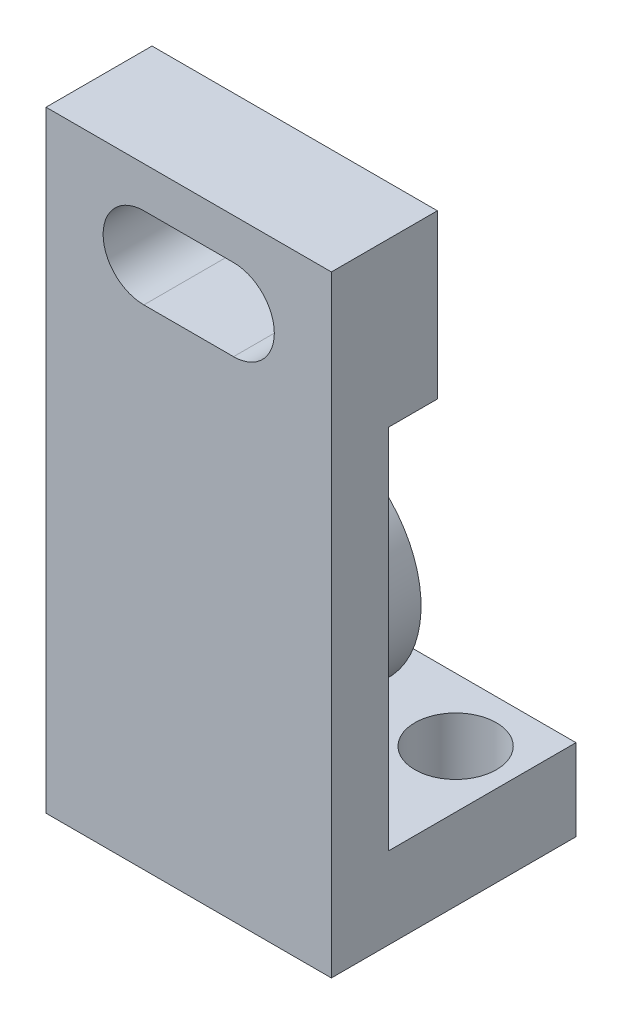
ISO-10303-21;
HEADER;
FILE_DESCRIPTION(('STEP AP214'),'2;1');
FILE_NAME('part.step','',(''),(''),'','','');
FILE_SCHEMA(('AUTOMOTIVE_DESIGN { 1 0 10303 214 1 1 1 1 }'));
ENDSEC;
DATA;
#1=APPLICATION_CONTEXT('core data for automotive mechanical design processes');
#2=APPLICATION_PROTOCOL_DEFINITION('international standard','automotive_design',2000,#1);
#3=PRODUCT_CONTEXT('',#1,'mechanical');
#4=PRODUCT('Part','Part','',(#3));
#5=PRODUCT_RELATED_PRODUCT_CATEGORY('part','',(#4));
#6=PRODUCT_DEFINITION_FORMATION('','',#4);
#7=PRODUCT_DEFINITION_CONTEXT('part definition',#1,'design');
#8=PRODUCT_DEFINITION('design','',#6,#7);
#9=PRODUCT_DEFINITION_SHAPE('','',#8);
#10=(LENGTH_UNIT() NAMED_UNIT(*) SI_UNIT(.MILLI.,.METRE.));
#11=(NAMED_UNIT(*) PLANE_ANGLE_UNIT() SI_UNIT($,.RADIAN.));
#12=(NAMED_UNIT(*) SI_UNIT($,.STERADIAN.) SOLID_ANGLE_UNIT());
#13=UNCERTAINTY_MEASURE_WITH_UNIT(LENGTH_MEASURE(1.E-05),#10,'distance_accuracy_value','');
#14=(GEOMETRIC_REPRESENTATION_CONTEXT(3) GLOBAL_UNCERTAINTY_ASSIGNED_CONTEXT((#13)) GLOBAL_UNIT_ASSIGNED_CONTEXT((#10,
#11,#12)) REPRESENTATION_CONTEXT('',''));
#15=CARTESIAN_POINT('',(0.,0.,0.));
#16=DIRECTION('',(0.,0.,1.));
#17=DIRECTION('',(1.,0.,0.));
#18=AXIS2_PLACEMENT_3D('',#15,#16,#17);
#19=CARTESIAN_POINT('',(17.5,9.99999999999999,-30.));
#20=DIRECTION('',(0.,-1.,0.));
#21=DIRECTION('',(0.,0.,-1.));
#22=AXIS2_PLACEMENT_3D('',#19,#20,#21);
#23=PLANE('',#22);
#24=CARTESIAN_POINT('',(-10.5,10.,-22.2406387747997));
#25=DIRECTION('',(0.,1.,0.));
#26=DIRECTION('',(0.,0.,1.));
#27=AXIS2_PLACEMENT_3D('',#24,#25,#26);
#28=CIRCLE('',#27,4.99999999999999);
#29=CARTESIAN_POINT('',(-10.5,10.,-17.2406387747997));
#30=VERTEX_POINT('',#29);
#31=EDGE_CURVE('E335',#30,#30,#28,.T.);
#32=ORIENTED_EDGE('',*,*,#31,.F.);
#33=EDGE_LOOP('',(#32));
#34=FACE_BOUND('',#33,.T.);
#35=CARTESIAN_POINT('',(10.5,10.,-22.2406387747997));
#36=DIRECTION('',(0.,1.,0.));
#37=DIRECTION('',(0.,0.,1.));
#38=AXIS2_PLACEMENT_3D('',#35,#36,#37);
#39=CIRCLE('',#38,4.99999999999999);
#40=CARTESIAN_POINT('',(10.5,10.,-17.2406387747997));
#41=VERTEX_POINT('',#40);
#42=EDGE_CURVE('E326',#41,#41,#39,.T.);
#43=ORIENTED_EDGE('',*,*,#42,.F.);
#44=EDGE_LOOP('',(#43));
#45=FACE_BOUND('',#44,.T.);
#46=DIRECTION('',(0.,0.,1.));
#47=VECTOR('',#46,1.);
#48=CARTESIAN_POINT('',(3.,9.99999999999999,-15.));
#49=LINE('',#48,#47);
#50=CARTESIAN_POINT('',(3.,9.99999999999999,-15.));
#51=VERTEX_POINT('',#50);
#52=CARTESIAN_POINT('',(3.,9.99999999999999,-7.));
#53=VERTEX_POINT('',#52);
#54=EDGE_CURVE('E158',#51,#53,#49,.T.);
#55=ORIENTED_EDGE('',*,*,#54,.T.);
#56=DIRECTION('',(-1.,0.,0.));
#57=VECTOR('',#56,1.);
#58=CARTESIAN_POINT('',(17.5,9.99999999999999,-7.));
#59=LINE('',#58,#57);
#60=CARTESIAN_POINT('',(17.5,9.99999999999999,-7.));
#61=VERTEX_POINT('',#60);
#62=EDGE_CURVE('E256',#61,#53,#59,.T.);
#63=ORIENTED_EDGE('',*,*,#62,.F.);
#64=DIRECTION('',(0.,0.,1.));
#65=VECTOR('',#64,1.);
#66=CARTESIAN_POINT('',(17.5,9.99999999999999,-30.));
#67=LINE('',#66,#65);
#68=CARTESIAN_POINT('',(17.5,9.99999999999999,-30.));
#69=VERTEX_POINT('',#68);
#70=EDGE_CURVE('E218',#69,#61,#67,.T.);
#71=ORIENTED_EDGE('',*,*,#70,.F.);
#72=DIRECTION('',(-1.,0.,0.));
#73=VECTOR('',#72,1.);
#74=CARTESIAN_POINT('',(17.5,9.99999999999999,-30.));
#75=LINE('',#74,#73);
#76=CARTESIAN_POINT('',(-17.5,9.99999999999999,-30.));
#77=VERTEX_POINT('',#76);
#78=EDGE_CURVE('E261',#69,#77,#75,.T.);
#79=ORIENTED_EDGE('',*,*,#78,.T.);
#80=DIRECTION('',(0.,0.,1.));
#81=VECTOR('',#80,1.);
#82=CARTESIAN_POINT('',(-17.5,9.99999999999999,-30.));
#83=LINE('',#82,#81);
#84=CARTESIAN_POINT('',(-17.5,9.99999999999999,-7.));
#85=VERTEX_POINT('',#84);
#86=EDGE_CURVE('E237',#77,#85,#83,.T.);
#87=ORIENTED_EDGE('',*,*,#86,.T.);
#88=CARTESIAN_POINT('',(-3.,9.99999999999999,-7.));
#89=VERTEX_POINT('',#88);
#90=EDGE_CURVE('E260',#89,#85,#59,.T.);
#91=ORIENTED_EDGE('',*,*,#90,.F.);
#92=DIRECTION('',(0.,0.,1.));
#93=VECTOR('',#92,1.);
#94=CARTESIAN_POINT('',(-3.,9.99999999999999,-15.));
#95=LINE('',#94,#93);
#96=CARTESIAN_POINT('',(-3.,9.99999999999999,-15.));
#97=VERTEX_POINT('',#96);
#98=EDGE_CURVE('E56',#97,#89,#95,.T.);
#99=ORIENTED_EDGE('',*,*,#98,.F.);
#100=DIRECTION('',(-1.,0.,0.));
#101=VECTOR('',#100,1.);
#102=CARTESIAN_POINT('',(3.,9.99999999999999,-15.));
#103=LINE('',#102,#101);
#104=EDGE_CURVE('E53',#51,#97,#103,.T.);
#105=ORIENTED_EDGE('',*,*,#104,.F.);
#106=EDGE_LOOP('',(#55,#63,#71,#79,#87,#91,#99,#105));
#107=FACE_BOUND('',#106,.T.);
#108=ADVANCED_FACE('F39',(#34,#45,#107),#23,.F.);
#109=CARTESIAN_POINT('',(17.5,75.,0.));
#110=DIRECTION('',(0.,0.,-1.));
#111=DIRECTION('',(0.,1.,0.));
#112=AXIS2_PLACEMENT_3D('',#109,#110,#111);
#113=PLANE('',#112);
#114=DIRECTION('',(1.,0.,0.));
#115=VECTOR('',#114,1.);
#116=CARTESIAN_POINT('',(17.5,70.,0.));
#117=LINE('',#116,#115);
#118=CARTESIAN_POINT('',(-5.5,70.,0.));
#119=VERTEX_POINT('',#118);
#120=CARTESIAN_POINT('',(5.5,70.,0.));
#121=VERTEX_POINT('',#120);
#122=EDGE_CURVE('E204',#119,#121,#117,.T.);
#123=ORIENTED_EDGE('',*,*,#122,.T.);
#124=CARTESIAN_POINT('',(5.5,65.,0.));
#125=DIRECTION('',(0.,0.,-1.));
#126=DIRECTION('',(0.,1.,0.));
#127=AXIS2_PLACEMENT_3D('',#124,#125,#126);
#128=CIRCLE('',#127,4.99999999999999);
#129=CARTESIAN_POINT('',(5.5,60.,0.));
#130=VERTEX_POINT('',#129);
#131=EDGE_CURVE('E210',#121,#130,#128,.T.);
#132=ORIENTED_EDGE('',*,*,#131,.T.);
#133=DIRECTION('',(-1.,0.,0.));
#134=VECTOR('',#133,1.);
#135=CARTESIAN_POINT('',(17.5,60.,0.));
#136=LINE('',#135,#134);
#137=CARTESIAN_POINT('',(-5.5,60.,0.));
#138=VERTEX_POINT('',#137);
#139=EDGE_CURVE('E195',#130,#138,#136,.T.);
#140=ORIENTED_EDGE('',*,*,#139,.T.);
#141=CARTESIAN_POINT('',(-5.5,65.,0.));
#142=DIRECTION('',(0.,0.,-1.));
#143=DIRECTION('',(0.,1.,0.));
#144=AXIS2_PLACEMENT_3D('',#141,#142,#143);
#145=CIRCLE('',#144,4.99999999999999);
#146=EDGE_CURVE('E203',#138,#119,#145,.T.);
#147=ORIENTED_EDGE('',*,*,#146,.T.);
#148=EDGE_LOOP('',(#123,#132,#140,#147));
#149=FACE_BOUND('',#148,.T.);
#150=DIRECTION('',(0.,-1.,0.));
#151=VECTOR('',#150,1.);
#152=CARTESIAN_POINT('',(-17.5,75.,0.));
#153=LINE('',#152,#151);
#154=CARTESIAN_POINT('',(-17.5,75.,0.));
#155=VERTEX_POINT('',#154);
#156=CARTESIAN_POINT('',(-17.5,0.,0.));
#157=VERTEX_POINT('',#156);
#158=EDGE_CURVE('E209',#155,#157,#153,.T.);
#159=ORIENTED_EDGE('',*,*,#158,.T.);
#160=DIRECTION('',(-1.,0.,0.));
#161=VECTOR('',#160,1.);
#162=CARTESIAN_POINT('',(17.5,0.,0.));
#163=LINE('',#162,#161);
#164=CARTESIAN_POINT('',(17.5,0.,0.));
#165=VERTEX_POINT('',#164);
#166=EDGE_CURVE('E11',#165,#157,#163,.T.);
#167=ORIENTED_EDGE('',*,*,#166,.F.);
#168=DIRECTION('',(0.,-1.,0.));
#169=VECTOR('',#168,1.);
#170=CARTESIAN_POINT('',(17.5,75.,0.));
#171=LINE('',#170,#169);
#172=CARTESIAN_POINT('',(17.5,75.,0.));
#173=VERTEX_POINT('',#172);
#174=EDGE_CURVE('E211',#173,#165,#171,.T.);
#175=ORIENTED_EDGE('',*,*,#174,.F.);
#176=DIRECTION('',(-1.,0.,0.));
#177=VECTOR('',#176,1.);
#178=CARTESIAN_POINT('',(17.5,75.,0.));
#179=LINE('',#178,#177);
#180=EDGE_CURVE('E228',#173,#155,#179,.T.);
#181=ORIENTED_EDGE('',*,*,#180,.T.);
#182=EDGE_LOOP('',(#159,#167,#175,#181));
#183=FACE_BOUND('',#182,.T.);
#184=ADVANCED_FACE('F41',(#149,#183),#113,.F.);
#185=CARTESIAN_POINT('',(17.5,0.,0.));
#186=DIRECTION('',(0.,1.,0.));
#187=DIRECTION('',(0.,0.,1.));
#188=AXIS2_PLACEMENT_3D('',#185,#186,#187);
#189=PLANE('',#188);
#190=CARTESIAN_POINT('',(-10.5,0.,-22.2406387747997));
#191=DIRECTION('',(0.,1.,0.));
#192=DIRECTION('',(0.,0.,1.));
#193=AXIS2_PLACEMENT_3D('',#190,#191,#192);
#194=CIRCLE('',#193,5.);
#195=CARTESIAN_POINT('',(-10.5,0.,-17.2406387747997));
#196=VERTEX_POINT('',#195);
#197=EDGE_CURVE('E328',#196,#196,#194,.T.);
#198=ORIENTED_EDGE('',*,*,#197,.T.);
#199=EDGE_LOOP('',(#198));
#200=FACE_BOUND('',#199,.T.);
#201=CARTESIAN_POINT('',(10.5,0.,-22.2406387747997));
#202=DIRECTION('',(0.,1.,0.));
#203=DIRECTION('',(0.,0.,1.));
#204=AXIS2_PLACEMENT_3D('',#201,#202,#203);
#205=CIRCLE('',#204,5.);
#206=CARTESIAN_POINT('',(10.5,0.,-17.2406387747997));
#207=VERTEX_POINT('',#206);
#208=EDGE_CURVE('E321',#207,#207,#205,.T.);
#209=ORIENTED_EDGE('',*,*,#208,.T.);
#210=EDGE_LOOP('',(#209));
#211=FACE_BOUND('',#210,.T.);
#212=DIRECTION('',(0.,0.,-1.));
#213=VECTOR('',#212,1.);
#214=CARTESIAN_POINT('',(-17.5,0.,0.));
#215=LINE('',#214,#213);
#216=CARTESIAN_POINT('',(-17.5,0.,-30.));
#217=VERTEX_POINT('',#216);
#218=EDGE_CURVE('E235',#157,#217,#215,.T.);
#219=ORIENTED_EDGE('',*,*,#218,.T.);
#220=DIRECTION('',(-1.,0.,0.));
#221=VECTOR('',#220,1.);
#222=CARTESIAN_POINT('',(17.5,0.,-30.));
#223=LINE('',#222,#221);
#224=CARTESIAN_POINT('',(17.5,0.,-30.));
#225=VERTEX_POINT('',#224);
#226=EDGE_CURVE('E50',#225,#217,#223,.T.);
#227=ORIENTED_EDGE('',*,*,#226,.F.);
#228=DIRECTION('',(0.,0.,-1.));
#229=VECTOR('',#228,1.);
#230=CARTESIAN_POINT('',(17.5,0.,0.));
#231=LINE('',#230,#229);
#232=EDGE_CURVE('E212',#165,#225,#231,.T.);
#233=ORIENTED_EDGE('',*,*,#232,.F.);
#234=ORIENTED_EDGE('',*,*,#166,.T.);
#235=EDGE_LOOP('',(#219,#227,#233,#234));
#236=FACE_BOUND('',#235,.T.);
#237=ADVANCED_FACE('F282',(#200,#211,#236),#189,.F.);
#238=CARTESIAN_POINT('',(17.5,0.,-30.));
#239=DIRECTION('',(0.,0.,1.));
#240=DIRECTION('',(1.,0.,0.));
#241=AXIS2_PLACEMENT_3D('',#238,#239,#240);
#242=PLANE('',#241);
#243=DIRECTION('',(0.,1.,0.));
#244=VECTOR('',#243,1.);
#245=CARTESIAN_POINT('',(-17.5,0.,-30.));
#246=LINE('',#245,#244);
#247=EDGE_CURVE('E234',#217,#77,#246,.T.);
#248=ORIENTED_EDGE('',*,*,#247,.T.);
#249=ORIENTED_EDGE('',*,*,#78,.F.);
#250=DIRECTION('',(0.,1.,0.));
#251=VECTOR('',#250,1.);
#252=CARTESIAN_POINT('',(17.5,0.,-30.));
#253=LINE('',#252,#251);
#254=EDGE_CURVE('E220',#225,#69,#253,.T.);
#255=ORIENTED_EDGE('',*,*,#254,.F.);
#256=ORIENTED_EDGE('',*,*,#226,.T.);
#257=EDGE_LOOP('',(#248,#249,#255,#256));
#258=FACE_BOUND('',#257,.T.);
#259=ADVANCED_FACE('F268',(#258),#242,.F.);
#260=CARTESIAN_POINT('',(17.5,9.99999999999999,-7.));
#261=DIRECTION('',(0.,0.,1.));
#262=DIRECTION('',(1.,0.,0.));
#263=AXIS2_PLACEMENT_3D('',#260,#261,#262);
#264=PLANE('',#263);
#265=DIRECTION('',(0.,-1.,0.));
#266=VECTOR('',#265,1.);
#267=CARTESIAN_POINT('',(3.,16.8375534189118,-7.));
#268=LINE('',#267,#266);
#269=CARTESIAN_POINT('',(3.,16.8375534189118,-7.));
#270=VERTEX_POINT('',#269);
#271=EDGE_CURVE('E301',#270,#53,#268,.T.);
#272=ORIENTED_EDGE('',*,*,#271,.F.);
#273=CARTESIAN_POINT('',(0.,30.,-7.));
#274=DIRECTION('',(0.,0.,-1.));
#275=DIRECTION('',(-1.,0.,0.));
#276=AXIS2_PLACEMENT_3D('',#273,#274,#275);
#277=CIRCLE('',#276,13.5);
#278=CARTESIAN_POINT('',(-3.,16.8375534189118,-7.));
#279=VERTEX_POINT('',#278);
#280=EDGE_CURVE('E175',#279,#270,#277,.T.);
#281=ORIENTED_EDGE('',*,*,#280,.F.);
#282=DIRECTION('',(0.,1.,0.));
#283=VECTOR('',#282,1.);
#284=CARTESIAN_POINT('',(-3.,16.8375534189118,-7.));
#285=LINE('',#284,#283);
#286=EDGE_CURVE('E168',#89,#279,#285,.T.);
#287=ORIENTED_EDGE('',*,*,#286,.F.);
#288=ORIENTED_EDGE('',*,*,#90,.T.);
#289=DIRECTION('',(0.,1.,0.));
#290=VECTOR('',#289,1.);
#291=CARTESIAN_POINT('',(-17.5,9.99999999999999,-7.));
#292=LINE('',#291,#290);
#293=CARTESIAN_POINT('',(-17.5,55.,-7.));
#294=VERTEX_POINT('',#293);
#295=EDGE_CURVE('E239',#85,#294,#292,.T.);
#296=ORIENTED_EDGE('',*,*,#295,.T.);
#297=DIRECTION('',(-1.,0.,0.));
#298=VECTOR('',#297,1.);
#299=CARTESIAN_POINT('',(17.5,55.,-7.));
#300=LINE('',#299,#298);
#301=CARTESIAN_POINT('',(17.5,55.,-7.));
#302=VERTEX_POINT('',#301);
#303=EDGE_CURVE('E255',#302,#294,#300,.T.);
#304=ORIENTED_EDGE('',*,*,#303,.F.);
#305=DIRECTION('',(0.,1.,0.));
#306=VECTOR('',#305,1.);
#307=CARTESIAN_POINT('',(17.5,9.99999999999999,-7.));
#308=LINE('',#307,#306);
#309=EDGE_CURVE('E222',#61,#302,#308,.T.);
#310=ORIENTED_EDGE('',*,*,#309,.F.);
#311=ORIENTED_EDGE('',*,*,#62,.T.);
#312=EDGE_LOOP('',(#272,#281,#287,#288,#296,#304,#310,#311));
#313=FACE_BOUND('',#312,.T.);
#314=ADVANCED_FACE('F305',(#313),#264,.F.);
#315=CARTESIAN_POINT('',(17.5,55.,-7.));
#316=DIRECTION('',(0.,1.,0.));
#317=DIRECTION('',(0.,0.,1.));
#318=AXIS2_PLACEMENT_3D('',#315,#316,#317);
#319=PLANE('',#318);
#320=DIRECTION('',(0.,0.,-1.));
#321=VECTOR('',#320,1.);
#322=CARTESIAN_POINT('',(-17.5,55.,-7.));
#323=LINE('',#322,#321);
#324=CARTESIAN_POINT('',(-17.5,55.,-13.));
#325=VERTEX_POINT('',#324);
#326=EDGE_CURVE('E244',#294,#325,#323,.T.);
#327=ORIENTED_EDGE('',*,*,#326,.T.);
#328=DIRECTION('',(-1.,0.,0.));
#329=VECTOR('',#328,1.);
#330=CARTESIAN_POINT('',(17.5,55.,-13.));
#331=LINE('',#330,#329);
#332=CARTESIAN_POINT('',(17.5,55.,-13.));
#333=VERTEX_POINT('',#332);
#334=EDGE_CURVE('E253',#333,#325,#331,.T.);
#335=ORIENTED_EDGE('',*,*,#334,.F.);
#336=DIRECTION('',(0.,0.,-1.));
#337=VECTOR('',#336,1.);
#338=CARTESIAN_POINT('',(17.5,55.,-7.));
#339=LINE('',#338,#337);
#340=EDGE_CURVE('E224',#302,#333,#339,.T.);
#341=ORIENTED_EDGE('',*,*,#340,.F.);
#342=ORIENTED_EDGE('',*,*,#303,.T.);
#343=EDGE_LOOP('',(#327,#335,#341,#342));
#344=FACE_BOUND('',#343,.T.);
#345=ADVANCED_FACE('F297',(#344),#319,.F.);
#346=CARTESIAN_POINT('',(17.5,55.,-13.));
#347=DIRECTION('',(0.,0.,1.));
#348=DIRECTION('',(1.,0.,0.));
#349=AXIS2_PLACEMENT_3D('',#346,#347,#348);
#350=PLANE('',#349);
#351=DIRECTION('',(-1.,0.,0.));
#352=VECTOR('',#351,1.);
#353=CARTESIAN_POINT('',(5.5,60.,-13.));
#354=LINE('',#353,#352);
#355=CARTESIAN_POINT('',(5.5,60.,-13.));
#356=VERTEX_POINT('',#355);
#357=CARTESIAN_POINT('',(-5.5,60.,-13.));
#358=VERTEX_POINT('',#357);
#359=EDGE_CURVE('E177',#356,#358,#354,.T.);
#360=ORIENTED_EDGE('',*,*,#359,.F.);
#361=CARTESIAN_POINT('',(5.5,65.,-13.));
#362=DIRECTION('',(0.,0.,-1.));
#363=DIRECTION('',(-1.,0.,0.));
#364=AXIS2_PLACEMENT_3D('',#361,#362,#363);
#365=CIRCLE('',#364,4.99999999999999);
#366=CARTESIAN_POINT('',(5.5,70.,-13.));
#367=VERTEX_POINT('',#366);
#368=EDGE_CURVE('E173',#367,#356,#365,.T.);
#369=ORIENTED_EDGE('',*,*,#368,.F.);
#370=DIRECTION('',(1.,0.,0.));
#371=VECTOR('',#370,1.);
#372=CARTESIAN_POINT('',(5.5,70.,-13.));
#373=LINE('',#372,#371);
#374=CARTESIAN_POINT('',(-5.5,70.,-13.));
#375=VERTEX_POINT('',#374);
#376=EDGE_CURVE('E189',#375,#367,#373,.T.);
#377=ORIENTED_EDGE('',*,*,#376,.F.);
#378=CARTESIAN_POINT('',(-5.5,65.,-13.));
#379=DIRECTION('',(0.,0.,-1.));
#380=DIRECTION('',(-1.,0.,0.));
#381=AXIS2_PLACEMENT_3D('',#378,#379,#380);
#382=CIRCLE('',#381,4.99999999999999);
#383=EDGE_CURVE('E181',#358,#375,#382,.T.);
#384=ORIENTED_EDGE('',*,*,#383,.F.);
#385=EDGE_LOOP('',(#360,#369,#377,#384));
#386=FACE_BOUND('',#385,.T.);
#387=DIRECTION('',(0.,1.,0.));
#388=VECTOR('',#387,1.);
#389=CARTESIAN_POINT('',(-17.5,55.,-13.));
#390=LINE('',#389,#388);
#391=CARTESIAN_POINT('',(-17.5,75.,-13.));
#392=VERTEX_POINT('',#391);
#393=EDGE_CURVE('E245',#325,#392,#390,.T.);
#394=ORIENTED_EDGE('',*,*,#393,.T.);
#395=DIRECTION('',(-1.,0.,0.));
#396=VECTOR('',#395,1.);
#397=CARTESIAN_POINT('',(17.5,75.,-13.));
#398=LINE('',#397,#396);
#399=CARTESIAN_POINT('',(17.5,75.,-13.));
#400=VERTEX_POINT('',#399);
#401=EDGE_CURVE('E248',#400,#392,#398,.T.);
#402=ORIENTED_EDGE('',*,*,#401,.F.);
#403=DIRECTION('',(0.,1.,0.));
#404=VECTOR('',#403,1.);
#405=CARTESIAN_POINT('',(17.5,55.,-13.));
#406=LINE('',#405,#404);
#407=EDGE_CURVE('E223',#333,#400,#406,.T.);
#408=ORIENTED_EDGE('',*,*,#407,.F.);
#409=ORIENTED_EDGE('',*,*,#334,.T.);
#410=EDGE_LOOP('',(#394,#402,#408,#409));
#411=FACE_BOUND('',#410,.T.);
#412=ADVANCED_FACE('F299',(#386,#411),#350,.F.);
#413=CARTESIAN_POINT('',(17.5,75.,-13.));
#414=DIRECTION('',(0.,-1.,0.));
#415=DIRECTION('',(0.,0.,-1.));
#416=AXIS2_PLACEMENT_3D('',#413,#414,#415);
#417=PLANE('',#416);
#418=DIRECTION('',(0.,0.,1.));
#419=VECTOR('',#418,1.);
#420=CARTESIAN_POINT('',(-17.5,75.,-13.));
#421=LINE('',#420,#419);
#422=EDGE_CURVE('E214',#392,#155,#421,.T.);
#423=ORIENTED_EDGE('',*,*,#422,.T.);
#424=ORIENTED_EDGE('',*,*,#180,.F.);
#425=DIRECTION('',(0.,0.,1.));
#426=VECTOR('',#425,1.);
#427=CARTESIAN_POINT('',(17.5,75.,-13.));
#428=LINE('',#427,#426);
#429=EDGE_CURVE('E226',#400,#173,#428,.T.);
#430=ORIENTED_EDGE('',*,*,#429,.F.);
#431=ORIENTED_EDGE('',*,*,#401,.T.);
#432=EDGE_LOOP('',(#423,#424,#430,#431));
#433=FACE_BOUND('',#432,.T.);
#434=ADVANCED_FACE('F292',(#433),#417,.F.);
#435=CARTESIAN_POINT('',(17.5,0.,0.));
#436=DIRECTION('',(1.,0.,0.));
#437=DIRECTION('',(0.,0.,-1.));
#438=AXIS2_PLACEMENT_3D('',#435,#436,#437);
#439=PLANE('',#438);
#440=ORIENTED_EDGE('',*,*,#174,.T.);
#441=ORIENTED_EDGE('',*,*,#232,.T.);
#442=ORIENTED_EDGE('',*,*,#254,.T.);
#443=ORIENTED_EDGE('',*,*,#70,.T.);
#444=ORIENTED_EDGE('',*,*,#309,.T.);
#445=ORIENTED_EDGE('',*,*,#340,.T.);
#446=ORIENTED_EDGE('',*,*,#407,.T.);
#447=ORIENTED_EDGE('',*,*,#429,.T.);
#448=EDGE_LOOP('',(#440,#441,#442,#443,#444,#445,#446,#447));
#449=FACE_BOUND('',#448,.T.);
#450=ADVANCED_FACE('F284',(#449),#439,.T.);
#451=CARTESIAN_POINT('',(-17.5,0.,0.));
#452=DIRECTION('',(1.,0.,0.));
#453=DIRECTION('',(0.,0.,-1.));
#454=AXIS2_PLACEMENT_3D('',#451,#452,#453);
#455=PLANE('',#454);
#456=ORIENTED_EDGE('',*,*,#158,.F.);
#457=ORIENTED_EDGE('',*,*,#422,.F.);
#458=ORIENTED_EDGE('',*,*,#393,.F.);
#459=ORIENTED_EDGE('',*,*,#326,.F.);
#460=ORIENTED_EDGE('',*,*,#295,.F.);
#461=ORIENTED_EDGE('',*,*,#86,.F.);
#462=ORIENTED_EDGE('',*,*,#247,.F.);
#463=ORIENTED_EDGE('',*,*,#218,.F.);
#464=EDGE_LOOP('',(#456,#457,#458,#459,#460,#461,#462,#463));
#465=FACE_BOUND('',#464,.T.);
#466=ADVANCED_FACE('F273',(#465),#455,.F.);
#467=CARTESIAN_POINT('',(5.5,65.,22.));
#468=DIRECTION('',(0.,0.,-1.));
#469=DIRECTION('',(-1.,0.,0.));
#470=AXIS2_PLACEMENT_3D('',#467,#468,#469);
#471=CYLINDRICAL_SURFACE('',#470,4.99999999999999);
#472=DIRECTION('',(0.,0.,-1.));
#473=VECTOR('',#472,1.);
#474=CARTESIAN_POINT('',(5.5,70.,22.));
#475=LINE('',#474,#473);
#476=EDGE_CURVE('E187',#121,#367,#475,.T.);
#477=ORIENTED_EDGE('',*,*,#476,.T.);
#478=ORIENTED_EDGE('',*,*,#368,.T.);
#479=DIRECTION('',(0.,0.,-1.));
#480=VECTOR('',#479,1.);
#481=CARTESIAN_POINT('',(5.5,60.,22.));
#482=LINE('',#481,#480);
#483=EDGE_CURVE('E188',#130,#356,#482,.T.);
#484=ORIENTED_EDGE('',*,*,#483,.F.);
#485=ORIENTED_EDGE('',*,*,#131,.F.);
#486=EDGE_LOOP('',(#477,#478,#484,#485));
#487=FACE_BOUND('',#486,.T.);
#488=ADVANCED_FACE('F374',(#487),#471,.F.);
#489=CARTESIAN_POINT('',(5.5,70.,22.));
#490=DIRECTION('',(0.,1.,0.));
#491=DIRECTION('',(0.,0.,1.));
#492=AXIS2_PLACEMENT_3D('',#489,#490,#491);
#493=PLANE('',#492);
#494=DIRECTION('',(0.,0.,-1.));
#495=VECTOR('',#494,1.);
#496=CARTESIAN_POINT('',(-5.5,70.,22.));
#497=LINE('',#496,#495);
#498=EDGE_CURVE('E193',#119,#375,#497,.T.);
#499=ORIENTED_EDGE('',*,*,#498,.T.);
#500=ORIENTED_EDGE('',*,*,#376,.T.);
#501=ORIENTED_EDGE('',*,*,#476,.F.);
#502=ORIENTED_EDGE('',*,*,#122,.F.);
#503=EDGE_LOOP('',(#499,#500,#501,#502));
#504=FACE_BOUND('',#503,.T.);
#505=ADVANCED_FACE('F371',(#504),#493,.F.);
#506=CARTESIAN_POINT('',(-5.5,65.,22.));
#507=DIRECTION('',(0.,0.,-1.));
#508=DIRECTION('',(-1.,0.,0.));
#509=AXIS2_PLACEMENT_3D('',#506,#507,#508);
#510=CYLINDRICAL_SURFACE('',#509,4.99999999999999);
#511=DIRECTION('',(0.,0.,-1.));
#512=VECTOR('',#511,1.);
#513=CARTESIAN_POINT('',(-5.5,60.,22.));
#514=LINE('',#513,#512);
#515=EDGE_CURVE('E191',#138,#358,#514,.T.);
#516=ORIENTED_EDGE('',*,*,#515,.T.);
#517=ORIENTED_EDGE('',*,*,#383,.T.);
#518=ORIENTED_EDGE('',*,*,#498,.F.);
#519=ORIENTED_EDGE('',*,*,#146,.F.);
#520=EDGE_LOOP('',(#516,#517,#518,#519));
#521=FACE_BOUND('',#520,.T.);
#522=ADVANCED_FACE('F372',(#521),#510,.F.);
#523=CARTESIAN_POINT('',(5.5,60.,22.));
#524=DIRECTION('',(0.,-1.,0.));
#525=DIRECTION('',(0.,0.,-1.));
#526=AXIS2_PLACEMENT_3D('',#523,#524,#525);
#527=PLANE('',#526);
#528=ORIENTED_EDGE('',*,*,#483,.T.);
#529=ORIENTED_EDGE('',*,*,#359,.T.);
#530=ORIENTED_EDGE('',*,*,#515,.F.);
#531=ORIENTED_EDGE('',*,*,#139,.F.);
#532=EDGE_LOOP('',(#528,#529,#530,#531));
#533=FACE_BOUND('',#532,.T.);
#534=ADVANCED_FACE('F365',(#533),#527,.F.);
#535=CARTESIAN_POINT('',(0.,30.,-15.));
#536=DIRECTION('',(0.,0.,-1.));
#537=DIRECTION('',(-1.,0.,0.));
#538=AXIS2_PLACEMENT_3D('',#535,#536,#537);
#539=PLANE('',#538);
#540=CARTESIAN_POINT('',(0.,30.,-15.));
#541=DIRECTION('',(0.,0.,-1.));
#542=DIRECTION('',(-1.,0.,0.));
#543=AXIS2_PLACEMENT_3D('',#540,#541,#542);
#544=CIRCLE('',#543,13.5);
#545=CARTESIAN_POINT('',(-3.,16.8375534189118,-15.));
#546=VERTEX_POINT('',#545);
#547=CARTESIAN_POINT('',(3.,16.8375534189118,-15.));
#548=VERTEX_POINT('',#547);
#549=EDGE_CURVE('E159',#546,#548,#544,.T.);
#550=ORIENTED_EDGE('',*,*,#549,.T.);
#551=DIRECTION('',(0.,-1.,0.));
#552=VECTOR('',#551,1.);
#553=CARTESIAN_POINT('',(3.,16.8375534189118,-15.));
#554=LINE('',#553,#552);
#555=EDGE_CURVE('E151',#548,#51,#554,.T.);
#556=ORIENTED_EDGE('',*,*,#555,.T.);
#557=ORIENTED_EDGE('',*,*,#104,.T.);
#558=DIRECTION('',(0.,1.,0.));
#559=VECTOR('',#558,1.);
#560=CARTESIAN_POINT('',(-3.,16.8375534189118,-15.));
#561=LINE('',#560,#559);
#562=EDGE_CURVE('E167',#97,#546,#561,.T.);
#563=ORIENTED_EDGE('',*,*,#562,.T.);
#564=EDGE_LOOP('',(#550,#556,#557,#563));
#565=FACE_BOUND('',#564,.T.);
#566=CARTESIAN_POINT('',(0.,30.,-15.));
#567=DIRECTION('',(0.,0.,-1.));
#568=DIRECTION('',(-1.,0.,0.));
#569=AXIS2_PLACEMENT_3D('',#566,#567,#568);
#570=CIRCLE('',#569,8.);
#571=CARTESIAN_POINT('',(-8.,30.,-15.));
#572=VERTEX_POINT('',#571);
#573=EDGE_CURVE('E314',#572,#572,#570,.T.);
#574=ORIENTED_EDGE('',*,*,#573,.F.);
#575=EDGE_LOOP('',(#574));
#576=FACE_BOUND('',#575,.T.);
#577=ADVANCED_FACE('F162',(#565,#576),#539,.T.);
#578=CARTESIAN_POINT('',(0.,30.,-15.));
#579=DIRECTION('',(0.,0.,1.));
#580=DIRECTION('',(1.,0.,0.));
#581=AXIS2_PLACEMENT_3D('',#578,#579,#580);
#582=CYLINDRICAL_SURFACE('',#581,13.5);
#583=ORIENTED_EDGE('',*,*,#280,.T.);
#584=DIRECTION('',(0.,0.,1.));
#585=VECTOR('',#584,1.);
#586=CARTESIAN_POINT('',(3.,16.8375534189118,-15.));
#587=LINE('',#586,#585);
#588=EDGE_CURVE('E156',#548,#270,#587,.T.);
#589=ORIENTED_EDGE('',*,*,#588,.F.);
#590=ORIENTED_EDGE('',*,*,#549,.F.);
#591=DIRECTION('',(0.,0.,1.));
#592=VECTOR('',#591,1.);
#593=CARTESIAN_POINT('',(-3.,16.8375534189118,-15.));
#594=LINE('',#593,#592);
#595=EDGE_CURVE('E309',#546,#279,#594,.T.);
#596=ORIENTED_EDGE('',*,*,#595,.T.);
#597=EDGE_LOOP('',(#583,#589,#590,#596));
#598=FACE_BOUND('',#597,.T.);
#599=ADVANCED_FACE('F171',(#598),#582,.T.);
#600=CARTESIAN_POINT('',(3.,16.8375534189118,-15.));
#601=DIRECTION('',(-1.,0.,0.));
#602=DIRECTION('',(0.,-1.,0.));
#603=AXIS2_PLACEMENT_3D('',#600,#601,#602);
#604=PLANE('',#603);
#605=ORIENTED_EDGE('',*,*,#271,.T.);
#606=ORIENTED_EDGE('',*,*,#54,.F.);
#607=ORIENTED_EDGE('',*,*,#555,.F.);
#608=ORIENTED_EDGE('',*,*,#588,.T.);
#609=EDGE_LOOP('',(#605,#606,#607,#608));
#610=FACE_BOUND('',#609,.T.);
#611=ADVANCED_FACE('F152',(#610),#604,.F.);
#612=CARTESIAN_POINT('',(-3.,16.8375534189118,-15.));
#613=DIRECTION('',(1.,0.,0.));
#614=DIRECTION('',(0.,1.,0.));
#615=AXIS2_PLACEMENT_3D('',#612,#613,#614);
#616=PLANE('',#615);
#617=ORIENTED_EDGE('',*,*,#286,.T.);
#618=ORIENTED_EDGE('',*,*,#595,.F.);
#619=ORIENTED_EDGE('',*,*,#562,.F.);
#620=ORIENTED_EDGE('',*,*,#98,.T.);
#621=EDGE_LOOP('',(#617,#618,#619,#620));
#622=FACE_BOUND('',#621,.T.);
#623=ADVANCED_FACE('F313',(#622),#616,.F.);
#624=CARTESIAN_POINT('',(0.,30.,-15.));
#625=DIRECTION('',(0.,0.,1.));
#626=DIRECTION('',(1.,0.,0.));
#627=AXIS2_PLACEMENT_3D('',#624,#625,#626);
#628=CYLINDRICAL_SURFACE('',#627,8.);
#629=ORIENTED_EDGE('',*,*,#573,.T.);
#630=EDGE_LOOP('',(#629));
#631=FACE_BOUND('',#630,.T.);
#632=CARTESIAN_POINT('',(0.,30.,-7.));
#633=DIRECTION('',(0.,0.,-1.));
#634=DIRECTION('',(-1.,0.,0.));
#635=AXIS2_PLACEMENT_3D('',#632,#633,#634);
#636=CIRCLE('',#635,8.);
#637=CARTESIAN_POINT('',(-8.,30.,-7.));
#638=VERTEX_POINT('',#637);
#639=EDGE_CURVE('E316',#638,#638,#636,.T.);
#640=ORIENTED_EDGE('',*,*,#639,.F.);
#641=EDGE_LOOP('',(#640));
#642=FACE_BOUND('',#641,.T.);
#643=ADVANCED_FACE('F352',(#631,#642),#628,.F.);
#644=ORIENTED_EDGE('',*,*,#639,.T.);
#645=EDGE_LOOP('',(#644));
#646=FACE_BOUND('',#645,.T.);
#647=ADVANCED_FACE('F341',(#646),#264,.F.);
#648=CARTESIAN_POINT('',(10.5,9.99999999999999,-22.2406387747997));
#649=DIRECTION('',(0.,1.,0.));
#650=DIRECTION('',(0.,0.,1.));
#651=AXIS2_PLACEMENT_3D('',#648,#649,#650);
#652=CYLINDRICAL_SURFACE('',#651,4.99999999999999);
#653=ORIENTED_EDGE('',*,*,#208,.F.);
#654=EDGE_LOOP('',(#653));
#655=FACE_BOUND('',#654,.T.);
#656=ORIENTED_EDGE('',*,*,#42,.T.);
#657=EDGE_LOOP('',(#656));
#658=FACE_BOUND('',#657,.T.);
#659=ADVANCED_FACE('F343',(#655,#658),#652,.F.);
#660=CARTESIAN_POINT('',(-10.5,9.99999999999999,-22.2406387747997));
#661=DIRECTION('',(0.,1.,0.));
#662=DIRECTION('',(0.,0.,1.));
#663=AXIS2_PLACEMENT_3D('',#660,#661,#662);
#664=CYLINDRICAL_SURFACE('',#663,4.99999999999999);
#665=ORIENTED_EDGE('',*,*,#197,.F.);
#666=EDGE_LOOP('',(#665));
#667=FACE_BOUND('',#666,.T.);
#668=ORIENTED_EDGE('',*,*,#31,.T.);
#669=EDGE_LOOP('',(#668));
#670=FACE_BOUND('',#669,.T.);
#671=ADVANCED_FACE('F339',(#667,#670),#664,.F.);
#672=CLOSED_SHELL('',(#108,#184,#237,#259,#314,#345,#412,#434,#450,#466,#488,#505,#522,#534,
#577,#599,#611,#623,#643,#647,#659,#671));
#673=MANIFOLD_SOLID_BREP('B2',#672);
#674=ADVANCED_BREP_SHAPE_REPRESENTATION('',(#18,#673),#14);
#675=SHAPE_DEFINITION_REPRESENTATION(#9,#674);
ENDSEC;
END-ISO-10303-21;
